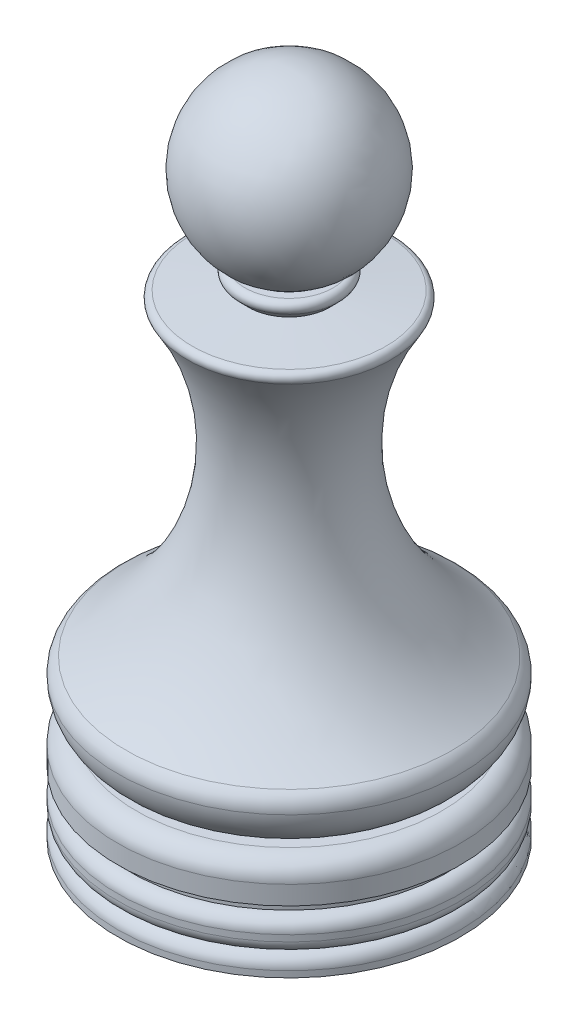
ISO-10303-21;
HEADER;
FILE_DESCRIPTION(('STEP AP214'),'2;1');
FILE_NAME('part.step','',(''),(''),'','','');
FILE_SCHEMA(('AUTOMOTIVE_DESIGN { 1 0 10303 214 1 1 1 1 }'));
ENDSEC;
DATA;
#1=APPLICATION_CONTEXT('core data for automotive mechanical design processes');
#2=APPLICATION_PROTOCOL_DEFINITION('international standard','automotive_design',2000,#1);
#3=PRODUCT_CONTEXT('',#1,'mechanical');
#4=PRODUCT('Part','Part','',(#3));
#5=PRODUCT_RELATED_PRODUCT_CATEGORY('part','',(#4));
#6=PRODUCT_DEFINITION_FORMATION('','',#4);
#7=PRODUCT_DEFINITION_CONTEXT('part definition',#1,'design');
#8=PRODUCT_DEFINITION('design','',#6,#7);
#9=PRODUCT_DEFINITION_SHAPE('','',#8);
#10=(LENGTH_UNIT() NAMED_UNIT(*) SI_UNIT(.MILLI.,.METRE.));
#11=(NAMED_UNIT(*) PLANE_ANGLE_UNIT() SI_UNIT($,.RADIAN.));
#12=(NAMED_UNIT(*) SI_UNIT($,.STERADIAN.) SOLID_ANGLE_UNIT());
#13=UNCERTAINTY_MEASURE_WITH_UNIT(LENGTH_MEASURE(1.E-05),#10,'distance_accuracy_value','');
#14=(GEOMETRIC_REPRESENTATION_CONTEXT(3) GLOBAL_UNCERTAINTY_ASSIGNED_CONTEXT((#13)) GLOBAL_UNIT_ASSIGNED_CONTEXT((#10,
#11,#12)) REPRESENTATION_CONTEXT('',''));
#15=CARTESIAN_POINT('',(0.,0.,0.));
#16=DIRECTION('',(0.,0.,1.));
#17=DIRECTION('',(1.,0.,0.));
#18=AXIS2_PLACEMENT_3D('',#15,#16,#17);
#19=CARTESIAN_POINT('',(0.,0.,0.));
#20=DIRECTION('',(0.,-1.,0.));
#21=DIRECTION('',(0.,0.,-1.));
#22=AXIS2_PLACEMENT_3D('',#19,#20,#21);
#23=PLANE('',#22);
#24=CARTESIAN_POINT('',(0.,0.,0.));
#25=DIRECTION('',(0.,-1.,0.));
#26=DIRECTION('',(0.,0.,-1.));
#27=AXIS2_PLACEMENT_3D('',#24,#25,#26);
#28=CIRCLE('',#27,27.5);
#29=CARTESIAN_POINT('',(0.,0.,-27.5));
#30=VERTEX_POINT('',#29);
#31=EDGE_CURVE('E42',#30,#30,#28,.T.);
#32=ORIENTED_EDGE('',*,*,#31,.T.);
#33=EDGE_LOOP('',(#32));
#34=FACE_BOUND('',#33,.T.);
#35=ADVANCED_FACE('F40',(#34),#23,.T.);
#36=CARTESIAN_POINT('',(0.,0.,0.));
#37=DIRECTION('',(0.,-1.,0.));
#38=DIRECTION('',(0.,0.,-1.));
#39=AXIS2_PLACEMENT_3D('',#36,#37,#38);
#40=CYLINDRICAL_SURFACE('',#39,27.5);
#41=CARTESIAN_POINT('',(0.,1.,0.));
#42=DIRECTION('',(0.,1.,0.));
#43=DIRECTION('',(0.,0.,1.));
#44=AXIS2_PLACEMENT_3D('',#41,#42,#43);
#45=CIRCLE('',#44,27.5);
#46=CARTESIAN_POINT('',(0.,1.,27.5));
#47=VERTEX_POINT('',#46);
#48=EDGE_CURVE('E10',#47,#47,#45,.F.);
#49=ORIENTED_EDGE('',*,*,#48,.T.);
#50=EDGE_LOOP('',(#49));
#51=FACE_BOUND('',#50,.T.);
#52=ORIENTED_EDGE('',*,*,#31,.F.);
#53=EDGE_LOOP('',(#52));
#54=FACE_BOUND('',#53,.T.);
#55=ADVANCED_FACE('F120',(#51,#54),#40,.T.);
#56=CARTESIAN_POINT('',(0.,5.,0.));
#57=DIRECTION('',(0.,-1.,0.));
#58=DIRECTION('',(0.,0.,-1.));
#59=AXIS2_PLACEMENT_3D('',#56,#57,#58);
#60=TOROIDAL_SURFACE('',#59,25.5,2.);
#61=CARTESIAN_POINT('',(0.,5.,0.));
#62=DIRECTION('',(0.,-1.,0.));
#63=DIRECTION('',(0.,0.,-1.));
#64=AXIS2_PLACEMENT_3D('',#61,#62,#63);
#65=CIRCLE('',#64,27.5);
#66=CARTESIAN_POINT('',(0.,5.,-27.5));
#67=VERTEX_POINT('',#66);
#68=EDGE_CURVE('E55',#67,#67,#65,.T.);
#69=ORIENTED_EDGE('',*,*,#68,.T.);
#70=EDGE_LOOP('',(#69));
#71=FACE_BOUND('',#70,.T.);
#72=CARTESIAN_POINT('',(0.,3.,0.));
#73=DIRECTION('',(0.,-1.,0.));
#74=DIRECTION('',(0.,0.,-1.));
#75=AXIS2_PLACEMENT_3D('',#72,#73,#74);
#76=CIRCLE('',#75,25.5);
#77=CARTESIAN_POINT('',(0.,3.,-25.5));
#78=VERTEX_POINT('',#77);
#79=EDGE_CURVE('E48',#78,#78,#76,.T.);
#80=ORIENTED_EDGE('',*,*,#79,.F.);
#81=EDGE_LOOP('',(#80));
#82=FACE_BOUND('',#81,.T.);
#83=ADVANCED_FACE('F124',(#71,#82),#60,.T.);
#84=CARTESIAN_POINT('',(0.,0.,0.));
#85=DIRECTION('',(0.,-1.,0.));
#86=DIRECTION('',(0.,0.,-1.));
#87=AXIS2_PLACEMENT_3D('',#84,#85,#86);
#88=CYLINDRICAL_SURFACE('',#87,27.5);
#89=CARTESIAN_POINT('',(0.,6.,0.));
#90=DIRECTION('',(0.,-1.,0.));
#91=DIRECTION('',(0.,0.,-1.));
#92=AXIS2_PLACEMENT_3D('',#89,#90,#91);
#93=CIRCLE('',#92,27.5);
#94=CARTESIAN_POINT('',(0.,6.,-27.5));
#95=VERTEX_POINT('',#94);
#96=EDGE_CURVE('E60',#95,#95,#93,.T.);
#97=ORIENTED_EDGE('',*,*,#96,.T.);
#98=EDGE_LOOP('',(#97));
#99=FACE_BOUND('',#98,.T.);
#100=ORIENTED_EDGE('',*,*,#68,.F.);
#101=EDGE_LOOP('',(#100));
#102=FACE_BOUND('',#101,.T.);
#103=ADVANCED_FACE('F127',(#99,#102),#88,.T.);
#104=CARTESIAN_POINT('',(0.,6.,0.));
#105=DIRECTION('',(0.,-1.,0.));
#106=DIRECTION('',(0.,0.,-1.));
#107=AXIS2_PLACEMENT_3D('',#104,#105,#106);
#108=TOROIDAL_SURFACE('',#107,25.5,2.);
#109=CARTESIAN_POINT('',(0.,8.,0.));
#110=DIRECTION('',(0.,-1.,0.));
#111=DIRECTION('',(0.,0.,-1.));
#112=AXIS2_PLACEMENT_3D('',#109,#110,#111);
#113=CIRCLE('',#112,25.5);
#114=CARTESIAN_POINT('',(0.,8.,-25.5));
#115=VERTEX_POINT('',#114);
#116=EDGE_CURVE('E58',#115,#115,#113,.T.);
#117=ORIENTED_EDGE('',*,*,#116,.T.);
#118=EDGE_LOOP('',(#117));
#119=FACE_BOUND('',#118,.T.);
#120=ORIENTED_EDGE('',*,*,#96,.F.);
#121=EDGE_LOOP('',(#120));
#122=FACE_BOUND('',#121,.T.);
#123=ADVANCED_FACE('F128',(#119,#122),#108,.T.);
#124=CARTESIAN_POINT('',(0.,0.,0.));
#125=DIRECTION('',(0.,-1.,0.));
#126=DIRECTION('',(0.,0.,-1.));
#127=AXIS2_PLACEMENT_3D('',#124,#125,#126);
#128=CYLINDRICAL_SURFACE('',#127,25.5);
#129=CARTESIAN_POINT('',(0.,10.,0.));
#130=DIRECTION('',(0.,-1.,0.));
#131=DIRECTION('',(0.,0.,-1.));
#132=AXIS2_PLACEMENT_3D('',#129,#130,#131);
#133=CIRCLE('',#132,25.5);
#134=CARTESIAN_POINT('',(0.,10.,-25.5));
#135=VERTEX_POINT('',#134);
#136=EDGE_CURVE('E65',#135,#135,#133,.T.);
#137=ORIENTED_EDGE('',*,*,#136,.T.);
#138=EDGE_LOOP('',(#137));
#139=FACE_BOUND('',#138,.T.);
#140=ORIENTED_EDGE('',*,*,#116,.F.);
#141=EDGE_LOOP('',(#140));
#142=FACE_BOUND('',#141,.T.);
#143=ADVANCED_FACE('F133',(#139,#142),#128,.T.);
#144=CARTESIAN_POINT('',(25.5,10.,0.));
#145=DIRECTION('',(0.,-1.,0.));
#146=DIRECTION('',(0.,0.,-1.));
#147=AXIS2_PLACEMENT_3D('',#144,#145,#146);
#148=PLANE('',#147);
#149=CARTESIAN_POINT('',(0.,10.,0.));
#150=DIRECTION('',(0.,-1.,0.));
#151=DIRECTION('',(0.,0.,-1.));
#152=AXIS2_PLACEMENT_3D('',#149,#150,#151);
#153=CIRCLE('',#152,27.5);
#154=CARTESIAN_POINT('',(0.,10.,-27.5));
#155=VERTEX_POINT('',#154);
#156=EDGE_CURVE('E68',#155,#155,#153,.T.);
#157=ORIENTED_EDGE('',*,*,#156,.T.);
#158=EDGE_LOOP('',(#157));
#159=FACE_BOUND('',#158,.T.);
#160=ORIENTED_EDGE('',*,*,#136,.F.);
#161=EDGE_LOOP('',(#160));
#162=FACE_BOUND('',#161,.T.);
#163=ADVANCED_FACE('F137',(#159,#162),#148,.T.);
#164=CARTESIAN_POINT('',(0.,0.,0.));
#165=DIRECTION('',(0.,-1.,0.));
#166=DIRECTION('',(0.,0.,-1.));
#167=AXIS2_PLACEMENT_3D('',#164,#165,#166);
#168=CYLINDRICAL_SURFACE('',#167,27.5);
#169=CARTESIAN_POINT('',(0.,13.,0.));
#170=DIRECTION('',(0.,-1.,0.));
#171=DIRECTION('',(0.,0.,-1.));
#172=AXIS2_PLACEMENT_3D('',#169,#170,#171);
#173=CIRCLE('',#172,27.5);
#174=CARTESIAN_POINT('',(0.,13.,-27.5));
#175=VERTEX_POINT('',#174);
#176=EDGE_CURVE('E70',#175,#175,#173,.T.);
#177=ORIENTED_EDGE('',*,*,#176,.T.);
#178=EDGE_LOOP('',(#177));
#179=FACE_BOUND('',#178,.T.);
#180=ORIENTED_EDGE('',*,*,#156,.F.);
#181=EDGE_LOOP('',(#180));
#182=FACE_BOUND('',#181,.T.);
#183=ADVANCED_FACE('F142',(#179,#182),#168,.T.);
#184=CARTESIAN_POINT('',(0.,13.,0.));
#185=DIRECTION('',(0.,-1.,0.));
#186=DIRECTION('',(0.,0.,-1.));
#187=AXIS2_PLACEMENT_3D('',#184,#185,#186);
#188=TOROIDAL_SURFACE('',#187,24.5,3.);
#189=CARTESIAN_POINT('',(0.,16.,0.));
#190=DIRECTION('',(0.,-1.,0.));
#191=DIRECTION('',(0.,0.,-1.));
#192=AXIS2_PLACEMENT_3D('',#189,#190,#191);
#193=CIRCLE('',#192,24.5);
#194=CARTESIAN_POINT('',(0.,16.,-24.5));
#195=VERTEX_POINT('',#194);
#196=EDGE_CURVE('E75',#195,#195,#193,.T.);
#197=ORIENTED_EDGE('',*,*,#196,.T.);
#198=EDGE_LOOP('',(#197));
#199=FACE_BOUND('',#198,.T.);
#200=ORIENTED_EDGE('',*,*,#176,.F.);
#201=EDGE_LOOP('',(#200));
#202=FACE_BOUND('',#201,.T.);
#203=ADVANCED_FACE('F148',(#199,#202),#188,.T.);
#204=CARTESIAN_POINT('',(24.5,16.,0.));
#205=DIRECTION('',(0.,1.,0.));
#206=DIRECTION('',(0.,0.,1.));
#207=AXIS2_PLACEMENT_3D('',#204,#205,#206);
#208=PLANE('',#207);
#209=CARTESIAN_POINT('',(0.,16.,0.));
#210=DIRECTION('',(0.,-1.,0.));
#211=DIRECTION('',(0.,0.,-1.));
#212=AXIS2_PLACEMENT_3D('',#209,#210,#211);
#213=CIRCLE('',#212,20.5);
#214=CARTESIAN_POINT('',(0.,16.,-20.5));
#215=VERTEX_POINT('',#214);
#216=EDGE_CURVE('E73',#215,#215,#213,.T.);
#217=ORIENTED_EDGE('',*,*,#216,.T.);
#218=EDGE_LOOP('',(#217));
#219=FACE_BOUND('',#218,.T.);
#220=ORIENTED_EDGE('',*,*,#196,.F.);
#221=EDGE_LOOP('',(#220));
#222=FACE_BOUND('',#221,.T.);
#223=ADVANCED_FACE('F147',(#219,#222),#208,.T.);
#224=CARTESIAN_POINT('',(0.,23.,0.));
#225=DIRECTION('',(0.,-1.,0.));
#226=DIRECTION('',(0.,0.,-1.));
#227=AXIS2_PLACEMENT_3D('',#224,#225,#226);
#228=TOROIDAL_SURFACE('',#227,20.5,7.);
#229=CARTESIAN_POINT('',(0.,22.6515809144338,0.));
#230=DIRECTION('',(0.,-1.,0.));
#231=DIRECTION('',(0.,0.,-1.));
#232=AXIS2_PLACEMENT_3D('',#229,#230,#231);
#233=CIRCLE('',#232,27.4913234899276);
#234=CARTESIAN_POINT('',(0.,22.6515809144338,-27.4913234899276));
#235=VERTEX_POINT('',#234);
#236=EDGE_CURVE('E80',#235,#235,#233,.T.);
#237=ORIENTED_EDGE('',*,*,#236,.T.);
#238=EDGE_LOOP('',(#237));
#239=FACE_BOUND('',#238,.T.);
#240=ORIENTED_EDGE('',*,*,#216,.F.);
#241=EDGE_LOOP('',(#240));
#242=FACE_BOUND('',#241,.T.);
#243=ADVANCED_FACE('F152',(#239,#242),#228,.T.);
#244=CARTESIAN_POINT('',(0.,22.8009033796765,0.));
#245=DIRECTION('',(0.,-1.,0.));
#246=DIRECTION('',(0.,0.,-1.));
#247=AXIS2_PLACEMENT_3D('',#244,#245,#246);
#248=TOROIDAL_SURFACE('',#247,24.4950419942443,3.);
#249=CARTESIAN_POINT('',(0.,25.2777569658552,0.));
#250=DIRECTION('',(0.,-1.,0.));
#251=DIRECTION('',(0.,0.,-1.));
#252=AXIS2_PLACEMENT_3D('',#249,#250,#251);
#253=CIRCLE('',#252,26.1877310716102);
#254=CARTESIAN_POINT('',(0.,25.2777569658552,-26.1877310716102));
#255=VERTEX_POINT('',#254);
#256=EDGE_CURVE('E83',#255,#255,#253,.T.);
#257=ORIENTED_EDGE('',*,*,#256,.T.);
#258=EDGE_LOOP('',(#257));
#259=FACE_BOUND('',#258,.T.);
#260=ORIENTED_EDGE('',*,*,#236,.F.);
#261=EDGE_LOOP('',(#260));
#262=FACE_BOUND('',#261,.T.);
#263=ADVANCED_FACE('F158',(#259,#262),#248,.T.);
#264=CARTESIAN_POINT('',(0.,55.,0.));
#265=DIRECTION('',(0.,-1.,0.));
#266=DIRECTION('',(0.,0.,-1.));
#267=AXIS2_PLACEMENT_3D('',#264,#265,#266);
#268=TOROIDAL_SURFACE('',#267,46.5,36.);
#269=CARTESIAN_POINT('',(0.,74.5887781509157,0.));
#270=DIRECTION('',(0.,-1.,0.));
#271=DIRECTION('',(0.,0.,-1.));
#272=AXIS2_PLACEMENT_3D('',#269,#270,#271);
#273=CIRCLE('',#272,16.2960305497074);
#274=CARTESIAN_POINT('',(0.,74.5887781509157,-16.2960305497074));
#275=VERTEX_POINT('',#274);
#276=EDGE_CURVE('E85',#275,#275,#273,.T.);
#277=ORIENTED_EDGE('',*,*,#276,.T.);
#278=EDGE_LOOP('',(#277));
#279=FACE_BOUND('',#278,.T.);
#280=ORIENTED_EDGE('',*,*,#256,.F.);
#281=EDGE_LOOP('',(#280));
#282=FACE_BOUND('',#281,.T.);
#283=ADVANCED_FACE('F165',(#279,#282),#268,.F.);
#284=CARTESIAN_POINT('',(0.,75.1329108773301,0.));
#285=DIRECTION('',(0.,-1.,0.));
#286=DIRECTION('',(0.,0.,-1.));
#287=AXIS2_PLACEMENT_3D('',#284,#285,#286);
#288=TOROIDAL_SURFACE('',#287,15.4570313983104,0.999999999999986);
#289=CARTESIAN_POINT('',(0.,76.1283070756972,0.));
#290=DIRECTION('',(0.,-1.,0.));
#291=DIRECTION('',(0.,0.,-1.));
#292=AXIS2_PLACEMENT_3D('',#289,#290,#291);
#293=CIRCLE('',#292,15.5528771508307);
#294=CARTESIAN_POINT('',(0.,76.1283070756972,-15.5528771508307));
#295=VERTEX_POINT('',#294);
#296=EDGE_CURVE('E87',#295,#295,#293,.T.);
#297=ORIENTED_EDGE('',*,*,#296,.T.);
#298=EDGE_LOOP('',(#297));
#299=FACE_BOUND('',#298,.T.);
#300=ORIENTED_EDGE('',*,*,#276,.F.);
#301=EDGE_LOOP('',(#300));
#302=FACE_BOUND('',#301,.T.);
#303=ADVANCED_FACE('F167',(#299,#302),#288,.T.);
#304=CARTESIAN_POINT('',(0.,76.1283070756972,0.));
#305=DIRECTION('',(0.,-1.,0.));
#306=DIRECTION('',(0.,0.,-1.));
#307=AXIS2_PLACEMENT_3D('',#304,#305,#306);
#308=CONICAL_SURFACE('',#307,15.5528771508307,1.4748032179352);
#309=CARTESIAN_POINT('',(0.,77.,0.));
#310=DIRECTION('',(0.,-1.,0.));
#311=DIRECTION('',(0.,0.,-1.));
#312=AXIS2_PLACEMENT_3D('',#309,#310,#311);
#313=CIRCLE('',#312,6.5);
#314=CARTESIAN_POINT('',(0.,77.,-6.5));
#315=VERTEX_POINT('',#314);
#316=EDGE_CURVE('E89',#315,#315,#313,.T.);
#317=ORIENTED_EDGE('',*,*,#316,.T.);
#318=EDGE_LOOP('',(#317));
#319=FACE_BOUND('',#318,.T.);
#320=ORIENTED_EDGE('',*,*,#296,.F.);
#321=EDGE_LOOP('',(#320));
#322=FACE_BOUND('',#321,.T.);
#323=ADVANCED_FACE('F168',(#319,#322),#308,.T.);
#324=CARTESIAN_POINT('',(0.,77.,0.));
#325=DIRECTION('',(0.,1.,0.));
#326=DIRECTION('',(0.,0.,1.));
#327=AXIS2_PLACEMENT_3D('',#324,#325,#326);
#328=CONICAL_SURFACE('',#327,6.5,0.781909916394351);
#329=CARTESIAN_POINT('',(0.,78.295364078908,0.));
#330=DIRECTION('',(0.,-1.,0.));
#331=DIRECTION('',(0.,0.,-1.));
#332=AXIS2_PLACEMENT_3D('',#329,#330,#331);
#333=CIRCLE('',#332,7.78635835683186);
#334=CARTESIAN_POINT('',(0.,78.295364078908,-7.78635835683186));
#335=VERTEX_POINT('',#334);
#336=EDGE_CURVE('E91',#335,#335,#333,.T.);
#337=ORIENTED_EDGE('',*,*,#336,.T.);
#338=EDGE_LOOP('',(#337));
#339=FACE_BOUND('',#338,.T.);
#340=ORIENTED_EDGE('',*,*,#316,.F.);
#341=EDGE_LOOP('',(#340));
#342=FACE_BOUND('',#341,.T.);
#343=ADVANCED_FACE('F173',(#339,#342),#328,.T.);
#344=CARTESIAN_POINT('',(0.,79.,0.));
#345=DIRECTION('',(0.,-1.,0.));
#346=DIRECTION('',(0.,0.,-1.));
#347=AXIS2_PLACEMENT_3D('',#344,#345,#346);
#348=TOROIDAL_SURFACE('',#347,7.07678931952343,0.999999999999996);
#349=CARTESIAN_POINT('',(0.,80.,0.));
#350=DIRECTION('',(0.,-1.,0.));
#351=DIRECTION('',(0.,0.,-1.));
#352=AXIS2_PLACEMENT_3D('',#349,#350,#351);
#353=CIRCLE('',#352,7.07678931952343);
#354=CARTESIAN_POINT('',(0.,80.,-7.07678931952343));
#355=VERTEX_POINT('',#354);
#356=EDGE_CURVE('E96',#355,#355,#353,.T.);
#357=ORIENTED_EDGE('',*,*,#356,.T.);
#358=EDGE_LOOP('',(#357));
#359=FACE_BOUND('',#358,.T.);
#360=ORIENTED_EDGE('',*,*,#336,.F.);
#361=EDGE_LOOP('',(#360));
#362=FACE_BOUND('',#361,.T.);
#363=ADVANCED_FACE('F113',(#359,#362),#348,.T.);
#364=CARTESIAN_POINT('',(7.07678931952343,80.,0.));
#365=DIRECTION('',(0.,1.,0.));
#366=DIRECTION('',(0.,0.,1.));
#367=AXIS2_PLACEMENT_3D('',#364,#365,#366);
#368=PLANE('',#367);
#369=CARTESIAN_POINT('',(0.,80.,0.));
#370=DIRECTION('',(0.,-1.,0.));
#371=DIRECTION('',(0.,0.,-1.));
#372=AXIS2_PLACEMENT_3D('',#369,#370,#371);
#373=CIRCLE('',#372,5.19615242270668);
#374=CARTESIAN_POINT('',(0.,80.,-5.19615242270668));
#375=VERTEX_POINT('',#374);
#376=EDGE_CURVE('E97',#375,#375,#373,.T.);
#377=ORIENTED_EDGE('',*,*,#376,.T.);
#378=EDGE_LOOP('',(#377));
#379=FACE_BOUND('',#378,.T.);
#380=ORIENTED_EDGE('',*,*,#356,.F.);
#381=EDGE_LOOP('',(#380));
#382=FACE_BOUND('',#381,.T.);
#383=ADVANCED_FACE('F103',(#379,#382),#368,.T.);
#384=CARTESIAN_POINT('',(0.,93.,0.));
#385=DIRECTION('',(0.,-1.,0.));
#386=DIRECTION('',(1.,0.,0.));
#387=AXIS2_PLACEMENT_3D('',#384,#385,#386);
#388=SPHERICAL_SURFACE('',#387,14.);
#389=ORIENTED_EDGE('',*,*,#376,.F.);
#390=EDGE_LOOP('',(#389));
#391=FACE_BOUND('',#390,.T.);
#392=ADVANCED_FACE('F106',(#391),#388,.T.);
#393=CARTESIAN_POINT('',(0.,1.,0.));
#394=DIRECTION('',(0.,1.,0.));
#395=DIRECTION('',(0.,0.,1.));
#396=AXIS2_PLACEMENT_3D('',#393,#394,#395);
#397=TOROIDAL_SURFACE('',#396,25.5,2.);
#398=ORIENTED_EDGE('',*,*,#79,.T.);
#399=EDGE_LOOP('',(#398));
#400=FACE_BOUND('',#399,.T.);
#401=ORIENTED_EDGE('',*,*,#48,.F.);
#402=EDGE_LOOP('',(#401));
#403=FACE_BOUND('',#402,.T.);
#404=ADVANCED_FACE('F39',(#400,#403),#397,.T.);
#405=CLOSED_SHELL('',(#35,#55,#83,#103,#123,#143,#163,#183,#203,#223,#243,#263,#283,#303,#323,
#343,#363,#383,#392,#404));
#406=MANIFOLD_SOLID_BREP('B2',#405);
#407=ADVANCED_BREP_SHAPE_REPRESENTATION('',(#18,#406),#14);
#408=SHAPE_DEFINITION_REPRESENTATION(#9,#407);
ENDSEC;
END-ISO-10303-21;
